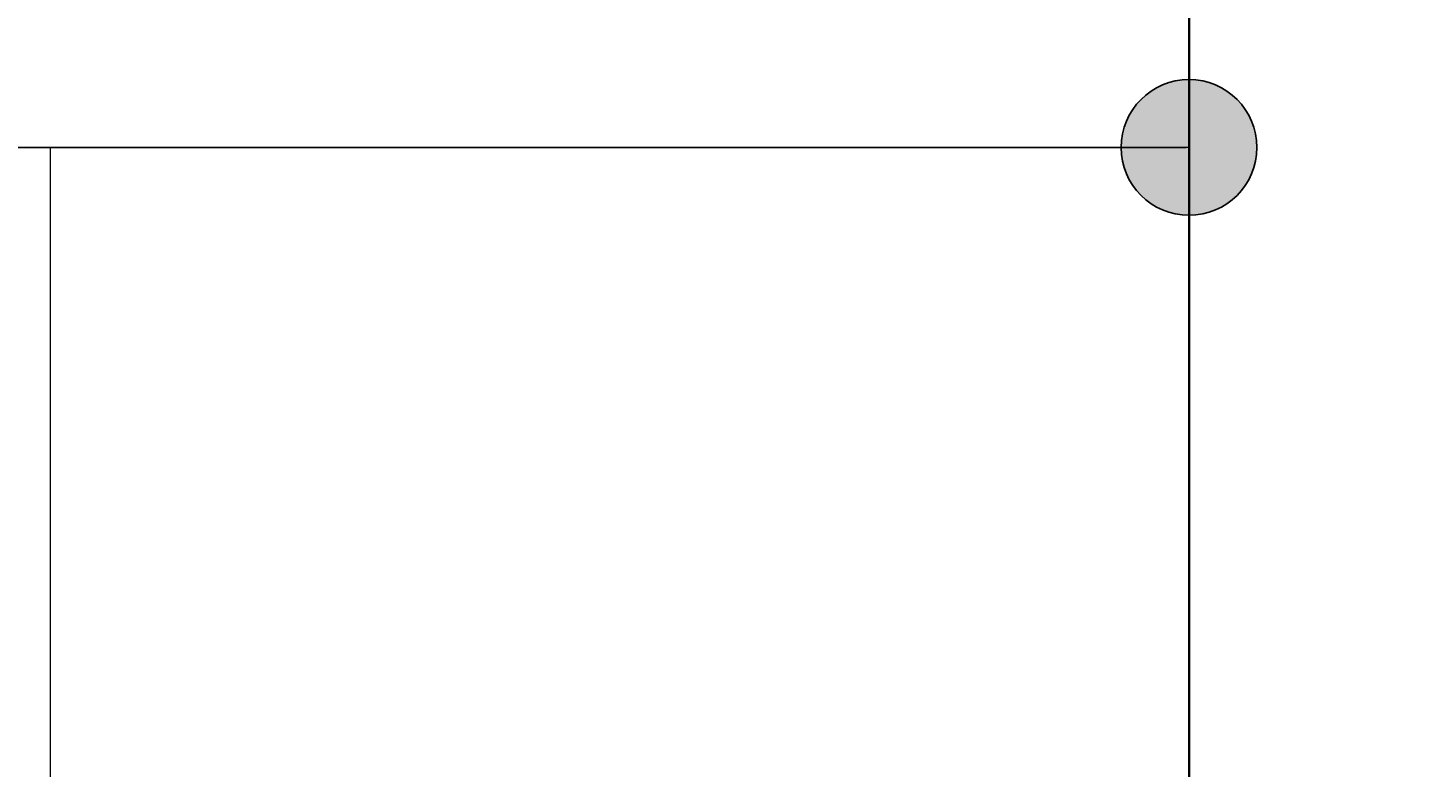
# Model space of a CAD drawing. Units: inches. Extents: x 738 to 1068, y 378 to 757.
# Tile 6 of 41: x 756 to 787, y 433 to 449. Entities that reach past the tile are written whole.
import ezdxf

# ---------------------------------------------------------------- set-up
doc = ezdxf.new("R2010")
doc.units = ezdxf.units.IN
doc.header["$MEASUREMENT"] = 0
for name, color, linetype, lineweight in [('A-ANNO-DIMS', 2, 'Continuous', 18), ('E-CONN', 7, 'Continuous', 25), ('E-CONN-PATT', 7, 'Continuous', 13), ('E-CTRL-WIRE', 7, 'Continuous', 18), ('E-POWR-FEED', 7, 'Continuous', 35)]:
    doc.layers.add(name, color=color, linetype=linetype, lineweight=lineweight)
doc.styles.get("Standard").update_dxf_attribs({"font": 'arial.ttf'})
doc.dimstyles.get("Standard").update_dxf_attribs({"dimtxt": 0.18, "dimasz": 0.18, "dimexe": 0.18, "dimexo": 0.0625, "dimgap": 0.09, "dimtad": 0, "dimtih": 1, "dimtoh": 1, "dimdec": 4, "dimzin": 0, "dimdsep": 46, "dimtxsty": 'Standard', "dimcen": 0.09, "dimadec": 0, "dimazin": 0, "dimtfac": 1, "dimtdec": 4, "dimtofl": 0, "dimtmove": 0, "dimatfit": 3, "dimfxl": 1, "dimtolj": 1, "dimtzin": 0, "dimarcsym": 0})

# ---------------------------------------------------------------- blocks, each defined once
blk = doc.blocks.new('*D19')
at = {"layer": 'A-ANNO-DIMS', "color": 0, "lineweight": -2, "transparency": 16777216}
for p, q in [((781.422, 446.265), (738.194, 446.265)), ((738.374, 446.085), (738.374, 421.499)), ((738.374, 396.549), (738.374, 421.135)), ((781.385, 396.369), (738.194, 396.369))]:
    blk.add_line(p, q, dxfattribs=at)
at = {"layer": 'A-ANNO-DIMS', "color": 0, "transparency": 16777216}
for points in [[(738.344, 446.085), (738.404, 446.085), (738.374, 446.265)], [(738.344, 396.549), (738.404, 396.549), (738.374, 396.369)]]:
    blk.add_solid(points, dxfattribs=at)
at = {"layer": 'Defpoints', "color": 0, "transparency": 16777216}
for p in [(738.374, 446.265), (781.485, 446.265), (781.447, 396.369)]:
    blk.add_point(p, dxfattribs=at)
at = {"layer": 'A-ANNO-DIMS', "color": 0, "transparency": 16777216, "insert": (738.374, 421.317), "char_height": 0.18, "attachment_point": 5}
blk.add_mtext('\\A1;49.9', dxfattribs=at)
blk = doc.blocks.new('*D20')
at = {"layer": 'A-ANNO-DIMS', "color": 0, "lineweight": -2, "transparency": 16777216}
for p, q in [((781.427, 461.392), (738.194, 461.392)), ((738.374, 461.212), (738.374, 454.01)), ((738.374, 446.445), (738.374, 453.647)), ((781.422, 446.265), (738.194, 446.265))]:
    blk.add_line(p, q, dxfattribs=at)
at = {"layer": 'A-ANNO-DIMS', "color": 0, "transparency": 16777216}
for points in [[(738.344, 461.212), (738.404, 461.212), (738.374, 461.392)], [(738.344, 446.445), (738.404, 446.445), (738.374, 446.265)]]:
    blk.add_solid(points, dxfattribs=at)
at = {"layer": 'Defpoints', "color": 0, "transparency": 16777216}
for p in [(738.374, 461.392), (781.49, 461.392), (781.485, 446.265)]:
    blk.add_point(p, dxfattribs=at)
at = {"layer": 'A-ANNO-DIMS', "color": 0, "transparency": 16777216, "insert": (738.374, 453.829), "char_height": 0.18, "attachment_point": 5}
blk.add_mtext('\\A1;15.127', dxfattribs=at)
blk = doc.blocks.new('*D25')
at = {"layer": 'A-ANNO-DIMS', "color": 0, "lineweight": -2, "transparency": 16777216}
for p, q in [((781.49, 646.923), (781.49, 378.239)), ((803.522, 646.923), (803.522, 378.239)), ((781.67, 378.419), (792.111, 378.419)), ((803.342, 378.419), (792.901, 378.419))]:
    blk.add_line(p, q, dxfattribs=at)
at = {"layer": 'A-ANNO-DIMS', "color": 0, "transparency": 16777216}
for points in [[(781.67, 378.449), (781.67, 378.389), (781.49, 378.419)], [(803.342, 378.449), (803.342, 378.389), (803.522, 378.419)]]:
    blk.add_solid(points, dxfattribs=at)
at = {"layer": 'Defpoints', "color": 0, "transparency": 16777216}
for p in [(781.49, 646.985), (803.522, 646.985), (803.522, 378.419)]:
    blk.add_point(p, dxfattribs=at)
at = {"layer": 'A-ANNO-DIMS', "color": 0, "transparency": 16777216, "insert": (792.506, 378.419), "char_height": 0.18, "attachment_point": 5}
blk.add_mtext('\\A1;22.03', dxfattribs=at)
blk = doc.blocks.new('*D34')
at = {"layer": 'A-ANNO-DIMS', "color": 0, "lineweight": -2, "transparency": 16777216}
for p, q in [((781.49, 686.266), (781.49, 378.239)), ((830.489, 686.266), (830.489, 378.239)), ((781.67, 378.419), (805.767, 378.419)), ((830.309, 378.419), (806.212, 378.419))]:
    blk.add_line(p, q, dxfattribs=at)
at = {"layer": 'A-ANNO-DIMS', "color": 0, "transparency": 16777216}
for points in [[(781.67, 378.449), (781.67, 378.389), (781.49, 378.419)], [(830.309, 378.449), (830.309, 378.389), (830.489, 378.419)]]:
    blk.add_solid(points, dxfattribs=at)
at = {"layer": 'Defpoints', "color": 0, "transparency": 16777216}
for p in [(781.49, 686.329), (830.489, 686.329), (830.489, 378.419)]:
    blk.add_point(p, dxfattribs=at)
at = {"layer": 'A-ANNO-DIMS', "color": 0, "transparency": 16777216, "insert": (805.99, 378.419), "char_height": 0.18, "attachment_point": 5}
blk.add_mtext('\\A1;49', dxfattribs=at)
blk = doc.blocks.new('*D38')
at = {"layer": 'A-ANNO-DIMS', "color": 0, "lineweight": -2, "transparency": 16777216}
for p, q in [((781.485, 593.017), (781.485, 378.239)), ((887.04, 593.067), (887.04, 378.239)), ((781.665, 378.419), (833.807, 378.419)), ((886.86, 378.419), (834.718, 378.419))]:
    blk.add_line(p, q, dxfattribs=at)
at = {"layer": 'A-ANNO-DIMS', "color": 0, "transparency": 16777216}
for points in [[(781.665, 378.449), (781.665, 378.389), (781.485, 378.419)], [(886.86, 378.449), (886.86, 378.389), (887.04, 378.419)]]:
    blk.add_solid(points, dxfattribs=at)
at = {"layer": 'Defpoints', "color": 0, "transparency": 16777216}
for p in [(781.485, 593.08), (887.04, 593.13), (887.04, 378.419)]:
    blk.add_point(p, dxfattribs=at)
at = {"layer": 'A-ANNO-DIMS', "color": 0, "transparency": 16777216, "insert": (834.263, 378.419), "char_height": 0.18, "attachment_point": 5}
blk.add_mtext('\\A1;105.56', dxfattribs=at)

msp = doc.modelspace()

# ---------------------------------------------------------------- hatches: boundary and pattern name
at = {"layer": 'E-CONN-PATT'}
h = msp.add_hatch(color=256, dxfattribs=at)
h.dxf.hatch_style = 1
h.paths.add_polyline_path([(782.9846, 446.2651, 0.4132247), (781.4897, 447.7651), (781.4897, 444.7651, 0.4132247)])
h.paths.add_polyline_path([(781.4897, 447.7651, 0.4152031), (779.9846, 446.2651, 0.4152031), (781.4897, 444.7651)])

# ---------------------------------------------------------------- linework, layer by layer
at = {"layer": 'E-CONN'}
msp.add_lwpolyline([(779.9846, 446.2651, 1), (782.9846, 446.2651, 1)], format="xyb", close=True, dxfattribs=at)
at = {"layer": 'E-CTRL-WIRE'}
for p, q in [((781.4846, 446.2651), (756.3236, 446.2651)), ((756.3236, 446.2651), (756.3236, 415.904))]:
    msp.add_line(p, q, dxfattribs=at)
at = {"layer": 'E-POWR-FEED'}
for p, q in [((781.4897, 686.329), (781.4897, 437.7164)), ((781.4897, 437.8486), (781.4897, 431.3208))]:
    msp.add_line(p, q, dxfattribs=at)

# ---------------------------------------------------------------- dimensions: what is measured, and where the dimension line sits
at = {"layer": 'A-ANNO-DIMS'}
for base, p1, p2, override, picture, middle in [((830.4893, 378.4191), (781.4897, 686.329), (830.4893, 686.329), {"dimdec": 0, "dimlfac": 1, "dimrnd": 0, "dimzin": 0, "dimdsep": 46, "dimlunit": 2}, '*D34', (805.9895, 378.4191)), ((803.5218, 378.4191), (781.4897, 646.9853), (803.5218, 646.9853), {"dimdec": 2, "dimlfac": 1, "dimrnd": 0, "dimzin": 0, "dimdsep": 46, "dimlunit": 2}, '*D25', (792.5057, 378.4191)), ((887.0404, 378.4191), (781.4846, 593.0796), (887.0404, 593.1296), {"dimdec": 2, "dimlfac": 1, "dimrnd": 0, "dimzin": 0, "dimdsep": 46, "dimlunit": 2}, '*D38', (834.2625, 378.4191))]:
    dim = msp.add_linear_dim(base=base, p1=p1, p2=p2, dimstyle='Standard', override=override, dxfattribs=at)
    dim.commit()
    dim.dimension.update_dxf_attribs({"geometry": picture, "text_midpoint": middle})
for base, p1, p2, override, picture, middle in [((738.3736, 461.3919), (781.4846, 446.2651), (781.4897, 461.3919), {"dimdec": 3, "dimlfac": 1, "dimrnd": 0, "dimzin": 0, "dimdsep": 46, "dimlunit": 2}, '*D20', (738.3736, 453.8285)), ((738.3736, 446.2651), (781.4474, 396.3691), (781.4846, 446.2651), {"dimdec": 1, "dimlfac": 1, "dimrnd": 0, "dimzin": 0, "dimdsep": 46, "dimlunit": 2}, '*D19', (738.3736, 421.3171))]:
    dim = msp.add_linear_dim(base=base, p1=p1, p2=p2, angle=90, dimstyle='Standard', override=override, dxfattribs=at)
    dim.commit()
    dim.dimension.update_dxf_attribs({"geometry": picture, "text_midpoint": middle})

doc.saveas('drawing.dxf')
